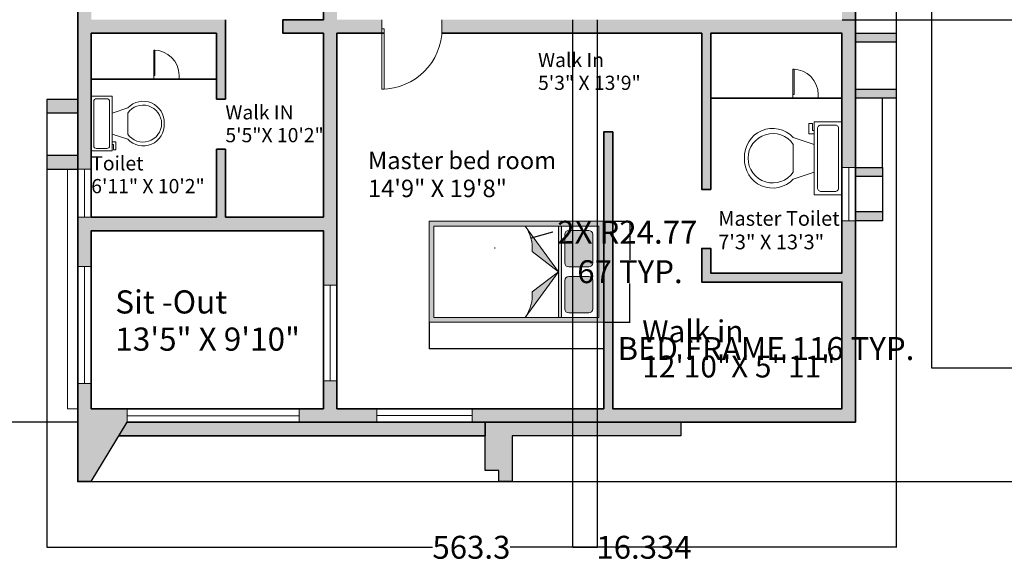
# Model space of a CAD drawing. Units: inches. Extents: x -828 to 1568, y -491 to 539.
# Tile 4 of 6: x 241 to 895, y -470 to -110. Entities that reach past the tile are written whole.
import ezdxf

# ---------------------------------------------------------------- set-up
doc = ezdxf.new("R2010")
doc.units = ezdxf.units.IN
doc.header["$MEASUREMENT"] = 0
doc.linetypes.add('ACAD_ISO02W100', pattern=[15, 12, -3])
for name, color, linetype, lineweight in [('A-ANNO-DIMS', 2, 'Continuous', 18), ('A-AREA-IDEN', 7, 'Continuous', 18), ('A-DOOR', 3, 'Continuous', 18), ('A-FLOR-EDGE', 7, 'Continuous', 25), ('A-FLOR-FIXT', 9, 'Continuous', 18), ('A-FLOR-OVHD', 116, 'ACAD_ISO02W100', 13), ('A-FLOR-SHFT', 7, 'Continuous', 25), ('A-FURN', 8, 'Continuous', 18), ('A-FURN-PATT', 253, 'Continuous', 13), ('A-GLAZ', 4, 'Continuous', 18), ('A-WALL', 7, 'Continuous', 35), ('A-WALL-PATT', 8, 'Continuous', 13)]:
    doc.layers.add(name, color=color, linetype=linetype, lineweight=lineweight)
doc.styles.get("Standard").update_dxf_attribs({"font": 'arial.ttf'})
doc.dimstyles.get("Standard").update_dxf_attribs({"dimtxt": 15.18, "dimasz": 0.18, "dimexe": 0.18, "dimexo": 0.0625, "dimgap": 0.09, "dimtad": 0, "dimtih": 1, "dimtoh": 1, "dimdec": 0, "dimzin": 0, "dimdsep": 46, "dimlunit": 3, "dimtxsty": 'Standard', "dimcen": 0.09, "dimadec": 0, "dimazin": 0, "dimtfac": 1, "dimtdec": 0, "dimtofl": 0, "dimtmove": 0, "dimatfit": 3, "dimfxl": 1, "dimtolj": 1, "dimtzin": 0, "dimarcsym": 0})

# ---------------------------------------------------------------- blocks, each defined once
blk = doc.blocks.new('*U2')
for p, q in [((0, 0), (0, -6)), ((40, 0), (40, -6))]:
    blk.add_line(p, q)
blk.add_lwpolyline([(0, 0), (0, 40), (1.75, 40), (1.75, 0)], close=True)
blk.add_arc((0, 0), 40, 0, 90)
blk = doc.blocks.new('*U6')
for p, q in [((9.5, -6), (9.5, -2)), ((-8, -8.5), (-8, -8)), ((-7, -8), (-7, -9.5)), ((-4, -8), (-6, -14)), ((4, -8), (6, -14)), ((-10, -8.5), (-8, -8.5)), ((-10, -9.5), (-10, -8.5)), ((-7, -9.5), (-10, -9.5)), ((4, -14), (-4, -14))]:
    blk.add_line(p, q)
blk.add_lwpolyline([(10.5, -8), (10.5, 0), (-10.5, 0), (-10.5, -8)], close=True)
for points in [[(-9.5, -2), (-9.5, -6)], [(8.5, -1), (-8.5, -1)], [(-8.5, -7), (8.5, -7)]]:
    blk.add_lwpolyline(points)
for centre, radius, start, end in [((-8.625, -1.875), 0.8839, 81.8699, 188.1301), ((8.625, -1.875), 0.8839, 351.8699, 98.1301), ((-8.625, -6.125), 0.8839, 171.869898, 278.1301), ((8.625, -6.125), 0.8839, 261.8699, 8.1301), ((-0.4772, -19.9188), 8.0953, 133.01722, 273.38), ((0.0374, -19.8731), 7.127, 124.50543, 269.7), ((-0.0373, -19.8731), 7.127, 270.3, 55.4946), ((0.4773, -19.9188), 8.0953, 266.62, 46.9828)]:
    blk.add_arc(centre, radius, start, end)
blk = doc.blocks.new('SERVICE-SHAFT-43')
blk.add_line((26.86, 37.12), (26.86, 6))
for points in [[(0, 43.12), (26.86, 43.12), (26.86, 37.12), (0, 37.12)], [(0, 6), (26.86, 6), (26.86, 0), (0, 0)]]:
    blk.add_lwpolyline(points, close=True)
blk = doc.blocks.new('BED-FRAME-TURNBACK')
h = blk.add_hatch(color=256)
h.dxf.hatch_style = 1
h.paths.add_polyline_path([(0, 0), (115.93, 0), (115.93, 67.12), (0, 67.12)])
h.paths.add_polyline_path([(3.27, 63.85), (112.66, 63.85), (112.66, 3.27), (3.27, 3.27)], flags=16)
h = blk.add_hatch(color=256)
h.dxf.hatch_style = 1
h.paths.add_polyline_path([(63.77, 63.85, -0.182673), (68.41, 46.96), (85.81, 33.56)])
h.paths.add_polyline_path([(85.81, 33.56), (68.41, 20.16, -0.182673), (63.77, 3.27)])
h = blk.add_hatch(color=256)
h.dxf.hatch_style = 1
h.paths.add_polyline_path([(87.78, 33.56), (85.81, 33.56), (85.81, 3.27), (87.78, 3.27)])
h.paths.add_polyline_path([(87.78, 63.85), (85.81, 63.85), (85.81, 33.56), (87.78, 33.56)])
for p, q in [((85.81, 33.56), (63.77, 63.85)), ((85.81, 3.27), (85.81, 63.85)), ((87.78, 3.27), (87.78, 63.85)), ((85.81, 33.56), (68.41, 46.96))]:
    blk.add_line(p, q)
for points in [[(115.93, 0), (0, 0), (0, 67.12), (115.93, 67.12)], [(112.66, 3.27), (3.27, 3.27), (3.27, 63.85), (112.66, 63.85)]]:
    blk.add_lwpolyline(points, close=True)
blk.add_lwpolyline([(63.77, 3.27, 0.182673), (68.41, 20.16), (85.81, 33.56)], format="xyb", close=True)
blk.add_arc((43.75, 49.27), 24.77, 354.63295, 36.04187)
blk = doc.blocks.new('*D29')
at = {"layer": 'A-ANNO-DIMS', "color": 0, "lineweight": -2, "transparency": 16777216}
for p, q in [((512.99, -311.15), (512.99, -328.66)), ((628.92, -311.15), (628.92, -328.66)), ((513.17, -328.48), (628.74, -328.48)), ((628.92, -328.48), (629.1, -328.48))]:
    blk.add_line(p, q, dxfattribs=at)
at = {"layer": 'A-ANNO-DIMS', "color": 0, "lineweight": 20, "transparency": 16777216}
for points in [[(513.17, -328.45), (513.17, -328.51), (512.99, -328.48)], [(628.74, -328.45), (628.74, -328.51), (628.92, -328.48)]]:
    blk.add_solid(points, dxfattribs=at)
at = {"layer": 'DEFPOINTS', "color": 0, "lineweight": 20, "transparency": 16777216}
for p in [(512.99, -311.09), (628.92, -311.09), (628.92, -328.48)]:
    blk.add_point(p, dxfattribs=at)
at = {"layer": 'A-ANNO-DIMS', "color": 0, "transparency": 16777216, "insert": (736.5, -328.48), "char_height": 15.18, "attachment_point": 5}
blk.add_mtext('\\A1;BED FRAME 116 TYP.', dxfattribs=at)
blk = doc.blocks.new('*D30')
at = {"layer": 'A-ANNO-DIMS', "color": 0, "lineweight": -2, "transparency": 16777216}
for p, q in [((628.99, -243.97), (646.49, -243.97)), ((646.31, -244.15), (646.31, -269.69)), ((646.31, -310.91), (646.31, -285.37)), ((628.99, -311.09), (646.49, -311.09))]:
    blk.add_line(p, q, dxfattribs=at)
at = {"layer": 'A-ANNO-DIMS', "color": 0, "lineweight": 20, "transparency": 16777216}
for points in [[(646.28, -244.15), (646.34, -244.15), (646.31, -243.97)], [(646.28, -310.91), (646.34, -310.91), (646.31, -311.09)]]:
    blk.add_solid(points, dxfattribs=at)
at = {"layer": 'DEFPOINTS', "color": 0, "lineweight": 20, "transparency": 16777216}
for p in [(628.92, -243.97), (646.31, -243.97), (628.92, -311.09)]:
    blk.add_point(p, dxfattribs=at)
at = {"layer": 'A-ANNO-DIMS', "color": 0, "transparency": 16777216, "insert": (646.31, -277.53), "char_height": 15.18, "attachment_point": 5}
blk.add_mtext('\\A1;67 TYP.', dxfattribs=at)
blk = doc.blocks.new('*D39')
at = {"layer": 'A-ANNO-DIMS', "color": 0, "lineweight": -2, "transparency": 16777216}
for p, q in [((822.78, -162.6), (822.78, -460.48)), ((259.43, -209.63), (259.43, -460.48)), ((259.61, -460.3), (515.4, -460.3)), ((822.6, -460.3), (566.81, -460.3))]:
    blk.add_line(p, q, dxfattribs=at)
at = {"layer": 'A-ANNO-DIMS', "color": 0, "lineweight": 20, "transparency": 16777216}
for points in [[(259.61, -460.27), (259.61, -460.33), (259.43, -460.3)], [(822.6, -460.27), (822.6, -460.33), (822.78, -460.3)]]:
    blk.add_solid(points, dxfattribs=at)
at = {"layer": 'DEFPOINTS', "color": 0, "lineweight": 20, "transparency": 16777216}
for p in [(822.78, -162.54), (259.43, -209.56), (822.78, -460.3)]:
    blk.add_point(p, dxfattribs=at)
at = {"layer": 'A-ANNO-DIMS', "color": 0, "transparency": 16777216, "insert": (541.11, -460.3), "char_height": 15.18, "attachment_point": 5}
blk.add_mtext('\\A1;563.3', dxfattribs=at)
blk = doc.blocks.new('*D40')
at = {"layer": 'A-ANNO-DIMS', "color": 0, "lineweight": -2, "transparency": 16777216}
for p, q in [((795.99, 360.63), (969.15, 360.63)), ((968.97, 360.45), (968.97, -20.38)), ((968.97, -416.57), (968.97, -35.74)), ((568.26, -416.75), (969.15, -416.75))]:
    blk.add_line(p, q, dxfattribs=at)
at = {"layer": 'A-ANNO-DIMS', "color": 0, "lineweight": 20, "transparency": 16777216}
for points in [[(968.94, 360.45), (969, 360.45), (968.97, 360.63)], [(968.94, -416.57), (969, -416.57), (968.97, -416.75)]]:
    blk.add_solid(points, dxfattribs=at)
at = {"layer": 'DEFPOINTS', "color": 0, "lineweight": 20, "transparency": 16777216}
for p in [(795.92, 360.63), (968.97, 360.63), (568.2, -416.75)]:
    blk.add_point(p, dxfattribs=at)
at = {"layer": 'A-ANNO-DIMS', "color": 0, "transparency": 16777216, "insert": (968.97, -28.06), "char_height": 15.18, "attachment_point": 5}
blk.add_mtext('\\A1;777.4', dxfattribs=at)
blk = doc.blocks.new('*D42')
at = {"layer": 'A-ANNO-DIMS', "color": 0, "lineweight": -2, "transparency": 16777216}
for p, q in [((347.86, 209.58), (141.48, 209.58)), ((141.66, 209.4), (141.66, -76.07)), ((141.66, -377.24), (141.66, -91.76)), ((279.86, -377.42), (141.48, -377.42))]:
    blk.add_line(p, q, dxfattribs=at)
at = {"layer": 'A-ANNO-DIMS', "color": 0, "lineweight": 20, "transparency": 16777216}
for points in [[(141.63, 209.4), (141.69, 209.4), (141.66, 209.58)], [(141.63, -377.24), (141.69, -377.24), (141.66, -377.42)]]:
    blk.add_solid(points, dxfattribs=at)
at = {"layer": 'DEFPOINTS', "color": 0, "lineweight": 20, "transparency": 16777216}
for p in [(141.66, 209.58), (347.92, 209.58), (279.92, -377.42)]:
    blk.add_point(p, dxfattribs=at)
at = {"layer": 'A-ANNO-DIMS', "color": 0, "transparency": 16777216, "insert": (141.66, -83.92), "char_height": 15.18, "attachment_point": 5}
blk.add_mtext('\\A1;587', dxfattribs=at)
blk = doc.blocks.new('*D47')
at = {"layer": 'A-ANNO-DIMS', "color": 0, "lineweight": -2, "transparency": 16777216}
for p, q in [((786.99, -22.42), (969.15, -22.42)), ((968.97, -22.6), (968.97, -58.57)), ((968.97, -110.24), (968.97, -74.26)), ((786.99, -110.42), (969.15, -110.42))]:
    blk.add_line(p, q, dxfattribs=at)
at = {"layer": 'A-ANNO-DIMS', "color": 0, "lineweight": 20, "transparency": 16777216}
for points in [[(968.94, -22.6), (969, -22.6), (968.97, -22.42)], [(968.94, -110.24), (969, -110.24), (968.97, -110.42)]]:
    blk.add_solid(points, dxfattribs=at)
at = {"layer": 'DEFPOINTS', "color": 0, "lineweight": 20, "transparency": 16777216}
for p in [(786.92, -22.42), (968.97, -22.42), (786.92, -110.42)]:
    blk.add_point(p, dxfattribs=at)
at = {"layer": 'A-ANNO-DIMS', "color": 0, "transparency": 16777216, "insert": (968.97, -66.42), "char_height": 15.18, "attachment_point": 5}
blk.add_mtext('\\A1;88', dxfattribs=at)
blk = doc.blocks.new('*D48')
at = {"layer": 'A-ANNO-DIMS', "color": 0, "lineweight": -2, "transparency": 16777216}
for p, q in [((608.26, -110.48), (608.26, -460.48)), ((624.59, -110.48), (624.59, -460.48)), ((608.44, -460.3), (624.41, -460.3)), ((624.59, -460.3), (624.77, -460.3))]:
    blk.add_line(p, q, dxfattribs=at)
at = {"layer": 'A-ANNO-DIMS', "color": 0, "lineweight": 20, "transparency": 16777216}
for points in [[(608.44, -460.27), (608.44, -460.33), (608.26, -460.3)], [(624.41, -460.27), (624.41, -460.33), (624.59, -460.3)]]:
    blk.add_solid(points, dxfattribs=at)
at = {"layer": 'DEFPOINTS', "color": 0, "lineweight": 20, "transparency": 16777216}
for p in [(608.26, -110.42), (624.59, -110.42), (624.59, -460.3)]:
    blk.add_point(p, dxfattribs=at)
at = {"layer": 'A-ANNO-DIMS', "color": 0, "transparency": 16777216, "insert": (655.62, -460.3), "char_height": 15.18, "attachment_point": 5}
blk.add_mtext('\\A1;16.334', dxfattribs=at)
blk = doc.blocks.new('*D54')
at = {"layer": 'A-ANNO-DIMS', "color": 0, "lineweight": -2, "transparency": 16777216}
for p, q in [((1093.6, 227.56), (846.26, 227.56)), ((846.44, 227.38), (846.44, -49.1)), ((846.44, -341.26), (846.44, -64.78)), ((1093.6, -341.44), (846.26, -341.44))]:
    blk.add_line(p, q, dxfattribs=at)
at = {"layer": 'A-ANNO-DIMS', "color": 0, "lineweight": 20, "transparency": 16777216}
for points in [[(846.41, 227.38), (846.47, 227.38), (846.44, 227.56)], [(846.41, -341.26), (846.47, -341.26), (846.44, -341.44)]]:
    blk.add_solid(points, dxfattribs=at)
at = {"layer": 'DEFPOINTS', "color": 0, "lineweight": 20, "transparency": 16777216}
for p in [(846.44, 227.56), (1093.66, 227.56), (1093.66, -341.44)]:
    blk.add_point(p, dxfattribs=at)
at = {"layer": 'A-ANNO-DIMS', "color": 0, "transparency": 16777216, "insert": (846.44, -56.94), "char_height": 15.18, "attachment_point": 5}
blk.add_mtext('\\A1;569', dxfattribs=at)
blk = doc.blocks.new('*D56')
at = {"layer": 'A-ANNO-DIMS', "color": 0, "lineweight": -2, "transparency": 16777216}
for p, q in [((594.95, -251.33), (580.8, -255.22)), ((595.13, -251.33), (594.95, -251.33)), ((556.64, -261.82), (556.82, -261.82)), ((556.73, -261.91), (556.73, -261.73))]:
    blk.add_line(p, q, dxfattribs=at)
at = {"layer": 'A-ANNO-DIMS', "color": 0, "lineweight": 20, "transparency": 16777216}
blk.add_solid([(580.79, -255.19), (580.8, -255.25), (580.62, -255.27)], dxfattribs=at)
at = {"layer": 'DEFPOINTS', "color": 0, "lineweight": 20, "transparency": 16777216}
for p in [(580.62, -255.27), (556.73, -261.82)]:
    blk.add_point(p, dxfattribs=at)
at = {"layer": 'A-ANNO-DIMS', "color": 0, "transparency": 16777216, "insert": (644.54, -251.33), "char_height": 15.18, "attachment_point": 5}
blk.add_mtext('\\A1;2X R24.77', dxfattribs=at)

msp = doc.modelspace()

# ---------------------------------------------------------------- hatches: boundary and pattern name
at = {"layer": 'A-FURN-PATT'}
h = msp.add_hatch(color=256, dxfattribs=at)
h.dxf.hatch_style = 1
h.paths.add_polyline_path([(621.5603, -252.8382, 0.41421356), (618.9442, -250.2221), (605.6981, -250.2221, 0.41421356), (603.0819, -252.8382), (603.0819, -271.7144, 0.41421356), (605.6981, -274.3306), (618.9442, -274.3306, 0.41421356), (621.5603, -271.7144)])
h = msp.add_hatch(color=256, dxfattribs=at)
h.dxf.hatch_style = 1
h.paths.add_polyline_path([(603.0819, -302.2257, 0.41421356), (605.6981, -304.8418), (618.9442, -304.8418, 0.41421356), (621.5603, -302.2257), (621.5603, -283.3495, 0.41421356), (618.9442, -280.7333), (605.6981, -280.7333, 0.41421356), (603.0819, -283.3495)])
at = {"layer": 'A-WALL-PATT'}
h = msp.add_hatch(color=256, dxfattribs=at)
h.dxf.hatch_style = 1
h.paths.add_polyline_path([(795.9226, -243.7164), (786.9226, -243.7164), (786.9226, -278.4155), (699.9226, -278.4155), (699.9226, -262.0576), (693.9226, -262.0576), (693.9226, -284.4155), (786.9226, -284.4155), (786.9226, -368.4155), (634.9226, -368.4155), (634.9226, -184.8338), (628.9226, -184.8338), (628.9226, -368.4155), (541.609, -368.4155), (541.609, -377.4155), (795.9226, -377.4155)])
h.paths.add_polyline_path([(795.9226, -80.4153), (786.9226, -80.4153), (786.9226, -110.4155), (521.5942, -110.4155), (521.5942, -116.4155, -0.01876983), (521.4815, -119.4155), (693.9226, -119.4155), (693.9226, -222.9922), (699.9226, -222.9922), (699.9226, -119.4155), (786.9226, -119.4155), (786.9226, -208.3743), (795.9226, -208.3743)])
h.paths.add_polyline_path([(822.7802, -119.4155), (795.9226, -119.4155), (795.9226, -125.4155), (822.7802, -125.4155)])
h.paths.add_polyline_path([(822.7802, -80.4153), (795.9226, -80.4153), (795.9226, -86.4153), (822.7802, -86.4153)])
h.paths.add_polyline_path([(822.7802, -156.5366), (795.9226, -156.5366), (795.9226, -162.5366), (822.7802, -162.5366)])
h.paths.add_polyline_path([(813.7802, -208.3743), (795.9226, -208.3743), (795.9226, -214.3743), (813.7802, -214.3743)])
h.paths.add_polyline_path([(813.7802, -237.7164), (795.9226, -237.7164), (795.9226, -243.7164), (813.7802, -243.7164)])
h.paths.add_polyline_path([(568.196, -386.4155), (680.1012, -386.4155), (680.1012, -377.4155), (550.196, -377.4155), (550.196, -409.2892), (559.196, -409.2892), (559.196, -416.7473), (568.196, -416.7473)])
h.paths.add_polyline_path([(478.3036, -368.4155), (451.9226, -368.4155), (451.9226, -349.8576), (442.9226, -349.8576), (442.9226, -368.4155), (426.7914, -368.4155), (426.7914, -377.4155), (478.3036, -377.4155)])
h.paths.add_polyline_path([(550.196, -377.4155), (541.609, -377.4155), (426.7914, -377.4155), (426.7914, -377.6482), (312.8078, -377.4155), (307.3423, -386.4155), (550.196, -386.4155)])
h.paths.add_polyline_path([(312.8078, -377.4155), (312.8078, -368.4155), (288.9226, -368.4155), (288.9226, -351.7781), (279.9226, -351.7781), (279.9226, -377.4155), (279.9226, -416.7473), (288.9226, -416.7473)])
h.paths.add_polyline_path([(451.9226, -119.4155), (481.5942, -119.4155), (481.5942, -116.4155), (481.5942, -110.4155), (451.9226, -110.4155), (451.9226, -5.2313), (445.9226, -5.2313, -0.01876983), (442.9226, -5.1187), (442.9226, -110.4155), (416.0227, -110.4155), (416.0227, -119.4155), (442.9226, -119.4155), (442.9226, -241.4155), (377.9226, -241.4155), (377.9226, -196.3369), (371.9226, -196.3369), (371.9226, -241.4155), (288.9226, -241.4155), (279.9226, -241.4155), (279.9226, -273.9916), (288.9226, -273.9916), (288.9226, -250.4155), (442.9226, -250.4155), (442.9226, -286.5741), (451.9226, -286.5741)])
h.paths.add_polyline_path([(377.9226, -110.4155), (288.9226, -110.4155), (288.9226, -23.5133), (279.9226, -23.5133), (279.9226, -209.5643), (288.9226, -209.5643), (288.9226, -119.4155), (371.9226, -119.4155), (371.9226, -163.1368), (377.9226, -163.1368)], flags=17)
h.paths.add_polyline_path([(279.9226, -200.5643), (259.4345, -200.5643), (259.4345, -209.5643), (279.9226, -209.5643)])
h.paths.add_polyline_path([(279.9226, -163.4155), (259.4345, -163.4155), (259.4345, -172.4155), (279.9226, -172.4155)])
h.paths.add_polyline_path([(680.9226, 59.5845), (569.9226, 59.5845), (569.9226, 238.5845), (603.4634, 238.5845), (603.4634, 244.5845), (569.9226, 244.5845), (569.9226, 333.5845), (663.9226, 333.5845), (663.9226, 280.6911), (667.9428, 280.6911, -0.00914136), (668.9226, 280.6732), (668.9226, 333.5845), (696.1553, 333.5845), (696.1553, 342.5845), (560.9226, 342.5845), (560.9226, 333.5845), (560.9226, 229.5845), (560.9226, 212.3675), (560.9226, 207.5845), (560.9226, 59.5845), (347.9226, 59.5845), (347.9226, 75.0877), (338.9226, 75.0877), (338.9226, 59.5845), (279.9226, 59.5845), (279.9226, 50.5845), (288.9226, 50.5845), (442.9226, 50.5845), (442.9226, 34.7687), (445.9226, 34.7687), (451.9226, 34.7687), (451.9226, 50.5845), (591.9226, 50.5845), (591.9226, 37.5639), (600.9226, 37.5639), (600.9226, 50.5845), (671.9226, 50.5845), (671.9226, -13.4155), (600.9226, -13.4155), (600.9226, -1.0868), (591.9226, -1.0868), (591.9226, -22.4155), (680.9226, -22.4155), (786.9226, -22.4155), (786.9226, -13.4155), (680.9226, -13.4155)])
h.paths.add_polyline_path([(813.7802, -22.4155), (795.9226, -22.4155), (795.9226, -28.4155), (813.7802, -28.4155)])
h.paths.add_polyline_path([(795.9226, 59.5845), (786.9226, 59.5845), (786.9226, -13.4155), (786.9226, -22.4155), (786.9226, -28.4155), (795.9226, -28.4155), (795.9226, -22.4155)])
h.paths.add_polyline_path([(813.7802, 16.5847), (795.9226, 16.5847), (795.9226, 10.5847), (813.7802, 10.5847)])
h.paths.add_polyline_path([(795.9226, 342.5845), (791.2302, 342.5845), (738.4317, 342.5845), (738.4317, 333.5845), (786.9226, 333.5845), (786.9226, 244.5845), (668.9226, 244.5845), (668.9226, 253.8895), (667.9428, 253.8895), (663.9226, 253.8895), (663.9226, 244.5845), (645.6004, 244.5845), (645.6004, 238.5845), (786.9226, 238.5845), (786.9226, 144.7189), (795.9226, 144.7189)])
h.paths.add_polyline_path([(822.7802, 207.4634), (795.9226, 207.4634), (795.9226, 201.4634), (822.7802, 201.4634)])
h.paths.add_polyline_path([(822.7802, 244.5845), (795.9226, 244.5845), (795.9226, 238.5845), (822.7802, 238.5845)])
h.paths.add_polyline_path([(347.9226, 207.5845), (386.8215, 207.5845), (485.9226, 207.5845), (485.9226, 229.5845), (489.9226, 229.5845), (489.9226, 244.2539), (489.9226, 333.5845), (521.5185, 333.5845), (521.5185, 342.5845), (279.9226, 342.5845), (279.9226, 333.5845), (338.9226, 333.5845), (347.9226, 333.5845), (483.9226, 333.5845), (483.9226, 209.5845), (386.8215, 209.5845), (338.9226, 209.5845), (279.9226, 209.5845), (279.9226, 200.5845), (288.9226, 200.5845), (338.9226, 200.5845), (338.9226, 180.8391), (347.9226, 180.8391)])
h.paths.add_polyline_path([(795.9226, 360.6319), (791.2302, 360.6319), (791.2302, 342.5845), (795.9226, 342.5845)])
h.paths.add_polyline_path([(755.2954, 360.6319), (750.6031, 360.6319), (750.6031, 342.5845), (755.2954, 342.5845)])
h.paths.add_polyline_path([(738.4317, 352.9518), (732.1778, 352.9518), (732.1778, 342.5845), (738.4317, 342.5845)])
h.paths.add_polyline_path([(702.4092, 352.9518), (696.1553, 352.9518), (696.1553, 342.5845), (702.4092, 342.5845)])
h.paths.add_polyline_path([(475.4018, 360.6319), (470.7095, 360.6319), (470.7095, 342.5845), (475.4018, 342.5845)])
h.paths.add_polyline_path([(448.7297, 360.6319), (444.0374, 360.6319), (444.0374, 342.5845), (448.7297, 342.5845)])
h.paths.add_polyline_path([(489.9226, 229.5845), (485.9226, 229.5845), (485.9226, 207.5845), (489.9226, 207.5845), (489.9226, 212.3675)], flags=17)
h.paths.add_polyline_path([(708.7018, -15.9815), (795.2211, -15.9815), (795.2211, -1.5493), (708.7018, -1.5493)], flags=9)
h.paths.add_polyline_path([(598.5172, 15.6725), (685.0365, 15.6725), (685.0365, 30.1047), (598.5172, 30.1047)], flags=25)
h.paths.add_polyline_path([(598.5188, 30.8165), (677.2194, 30.8165), (677.2194, 45.2391), (598.5188, 45.2391)], flags=25)

# ---------------------------------------------------------------- linework, layer by layer
at = {"layer": 'A-FLOR-EDGE'}
for p, q in [((288.9226, -416.7473), (312.8078, -377.4155)), ((550.196, -409.2892), (550.196, -377.4155)), ((559.196, -409.2892), (550.196, -409.2892)), ((559.196, -416.7473), (559.196, -409.2892)), ((288.9226, -416.7473), (568.196, -416.7473)), ((568.196, -416.7473), (559.196, -416.7473))]:
    msp.add_line(p, q, dxfattribs=at)
for points in [[(550.196, -377.4155), (550.196, -386.4155)], [(307.3423, -386.4155), (550.196, -386.4155)]]:
    msp.add_lwpolyline(points, close=True, dxfattribs=at)
msp.add_lwpolyline([(680.1012, -377.4155), (680.1012, -386.4155), (568.196, -386.4155), (568.196, -416.7473)], dxfattribs=at)
at = {"layer": 'A-FLOR-OVHD'}
msp.add_lwpolyline([(273.1806, -368.4155), (273.1806, -209.5643), (273.1806, -368.4155), (279.9226, -368.4155)], dxfattribs=at)
at = {"layer": 'A-FLOR-SHFT'}
for p, q in [((822.7802, -86.4153), (822.7802, -119.4155)), ((813.7802, -208.3743), (813.7802, -162.5366)), ((279.9226, -200.5643), (259.4345, -200.5643)), ((813.7802, -214.3743), (813.7802, -237.7164))]:
    msp.add_line(p, q, dxfattribs=at)
for points in [[(279.9226, -163.4155), (259.4345, -163.4155), (259.4345, -172.4155)], [(279.9226, -172.4155), (259.4345, -172.4155), (259.4345, -200.5643), (259.4345, -209.5643), (279.9226, -209.5643)], [(786.9226, -214.3743), (786.9226, -208.3743)], [(795.9226, -208.3743), (813.7802, -208.3743), (813.7802, -214.3743), (795.9226, -214.3743)], [(786.9226, -243.7164), (786.9226, -237.7164)], [(795.9226, -237.7164), (813.7802, -237.7164), (813.7802, -243.7164), (795.9226, -243.7164)]]:
    msp.add_lwpolyline(points, dxfattribs=at)
at = {"layer": 'A-FURN'}
for points in [[(618.9442, -274.3306), (605.6981, -274.3306, -0.41421356), (603.0819, -271.7144), (603.0819, -252.8382, -0.41421356), (605.6981, -250.2221), (618.9442, -250.2221, -0.41421356), (621.5603, -252.8382), (621.5603, -271.7144, -0.41421356)], [(618.9442, -280.7333), (605.6981, -280.7333, 0.41421356), (603.0819, -283.3495), (603.0819, -302.2257, 0.41421356), (605.6981, -304.8418), (618.9442, -304.8418, 0.41421356), (621.5603, -302.2257), (621.5603, -283.3495, 0.41421356)]]:
    msp.add_lwpolyline(points, format="xyb", close=True, dxfattribs=at)
at = {"layer": 'A-GLAZ'}
for p, q in [((791.4226, -243.7164), (791.4226, -208.3743)), ((284.4226, -241.4155), (284.4226, -209.5643)), ((284.4226, -351.7781), (284.4226, -273.9916)), ((447.4226, -349.8576), (447.4226, -286.5741)), ((426.7914, -373.1482), (312.8078, -373.1482)), ((541.609, -372.9155), (478.3036, -372.9155))]:
    msp.add_line(p, q, dxfattribs=at)
for points in [[(795.9226, -243.7164), (786.9226, -243.7164), (786.9226, -208.3743), (795.9226, -208.3743)], [(288.9226, -241.4155), (279.9226, -241.4155), (279.9226, -209.5643), (288.9226, -209.5643)], [(288.9226, -351.7781), (279.9226, -351.7781), (279.9226, -273.9916), (288.9226, -273.9916)], [(451.9226, -349.8576), (442.9226, -349.8576), (442.9226, -286.5741), (451.9226, -286.5741)], [(312.8078, -377.4155), (426.7914, -377.6482), (426.7914, -368.6482), (312.8078, -368.4155)], [(478.3036, -368.4155), (541.609, -368.4155), (541.609, -377.4155), (478.3036, -377.4155)]]:
    msp.add_lwpolyline(points, close=True, dxfattribs=at)
at = {"layer": 'A-WALL'}
for p, q in [((795.9226, 342.5845), (795.9226, -377.4155)), ((377.9226, -163.1368), (377.9226, -110.4155)), ((288.9226, -119.4155), (371.9226, -119.4155)), ((288.9226, -119.4155), (288.9226, -241.4155)), ((288.9226, -241.4155), (288.9226, -119.4155)), ((371.9226, -163.1368), (371.9226, -119.4155)), ((442.9226, -119.4155), (442.9226, -241.4155)), ((288.9226, -149.8674), (371.9226, -149.8674)), ((699.9226, -162.5366), (786.9226, -162.5366)), ((371.9226, -241.4155), (371.9226, -196.3369)), ((377.9226, -241.4155), (377.9226, -196.3369)), ((288.9226, -241.4155), (371.9226, -241.4155)), ((377.9226, -241.4155), (442.9226, -241.4155)), ((312.8078, -377.4155), (795.9226, -377.4155))]:
    msp.add_line(p, q, dxfattribs=at)
for points in [[(279.9226, 333.5845), (279.9226, 342.5845), (279.9226, 50.5845), (279.9226, -377.4155), (279.9226, -416.7473), (288.9226, -416.7473)], [(442.9226, -241.4155), (442.9226, -119.4155), (416.0227, -119.4155), (416.0227, -110.4155), (442.9226, -110.4155), (442.9226, -5.1187)], [(786.9226, -119.4155), (699.9226, -119.4155), (786.9226, -119.4155), (786.9226, -278.4155), (699.9226, -278.4155), (699.9226, -262.0576), (693.9226, -262.0576), (693.9226, -284.4155), (786.9226, -284.4155), (786.9226, -368.4155), (634.9226, -368.4155), (634.9226, -184.8338), (628.9226, -184.8338), (628.9226, -368.4155), (451.9226, -368.4155), (451.9226, -119.4155), (483.3442, -119.4155)], [(521.4815, -119.4155), (693.9226, -119.4155), (693.9226, -222.9922), (699.9226, -222.9922), (699.9226, -119.4155)], [(371.9226, -163.1368), (377.9226, -163.1368)], [(377.9226, -196.3369), (371.9226, -196.3369)]]:
    msp.add_lwpolyline(points, dxfattribs=at)
msp.add_lwpolyline([(288.9226, -368.4155), (442.9226, -368.4155), (442.9226, -250.4155), (288.9226, -250.4155)], close=True, dxfattribs=at)

# ---------------------------------------------------------------- block references
at = {"layer": 'A-DOOR', "xscale": -1, "rotation": 180}
msp.add_blockref('*U2', (481.5942, -116.4155), dxfattribs=at)
at = {"layer": 'A-DOOR', "xscale": 0.4187164315817437, "yscale": 0.4187164315817437, "zscale": 0.4187164315817437}
for p in [(330.4226, -147.3551), (754.4226, -160.0243)]:
    msp.add_blockref('*U2', p, dxfattribs=at)
at = {"layer": 'A-FLOR-FIXT'}
for p, xscale, yscale, zscale, rotation in [((288.9226, -179.3229), 1.728531319999881, 1.728531319999881, 1.728531319999881, 90), ((786.9226, -202.3123), 2.308307865517238, 2.308307865517238, 2.308307865517238, 270)]:
    msp.add_blockref('*U6', p, dxfattribs=dict(at, xscale=xscale, yscale=yscale, zscale=zscale, rotation=rotation))
at = {"layer": 'A-FLOR-SHFT'}
msp.add_blockref('SERVICE-SHAFT-43', (795.923, -162.537), dxfattribs=at)
at = {"layer": 'A-FURN'}
msp.add_blockref('BED-FRAME-TURNBACK', (512.989, -311.0915), dxfattribs=at)

# ---------------------------------------------------------------- texts
at = {"layer": 'A-AREA-IDEN'}
for s, height, p in [('Walk In', 9.42222, (585.3115, -141.8405)), ('5\'3" X 13\'9"', 9.422225, (585.3115, -156.9765)), ('Walk IN', 9.42222, (377.9226, -176.5448)), ('5\'5"X 10\'2"', 9.422225, (377.9226, -191.6808)), ('Toilet ', 9.42222, (288.9226, -210.3539)), ('Master bed room', 11.542757, (472.4915, -209.5342)), ('6\'11" X 10\'2"', 9.422225, (288.9226, -225.4899)), ('14\'9" X 19\'8"', 11.542757, (472.4915, -228.0766)), ('Master Toilet', 9.717003, (704.8376, -247.0736)), ('7\'3" X 13\'3"', 9.717003, (704.8376, -262.6831)), ('Sit -Out', 15.34207, (304.876, -305.2596)), ('Walk in', 14.539, (654.4439, -324.3313)), ('13\'5" X 9\'10"', 15.34207, (304.876, -329.9053)), ('12\'10"X 5\'\'11"', 14.538996, (654.4439, -347.687))]:
    msp.add_text(s, height=height, dxfattribs=at).set_placement(p)

# ---------------------------------------------------------------- dimensions: what is measured, and where the dimension line sits
at = {"layer": 'A-ANNO-DIMS'}
for base, p1, p2, override, picture, middle in [((968.971, 360.6319), (568.196, -416.7473), (795.9226, 360.6319), {"dimdec": 1, "dimlfac": 1, "dimrnd": 0, "dimzin": 0, "dimdsep": 46, "dimlunit": 2}, '*D40', (968.971, -28.0577)), ((846.4381, 227.5603), (1093.6584, -341.4397), (1093.6584, 227.5603), {"dimdec": 0, "dimlfac": 1, "dimrnd": 0, "dimzin": 0, "dimdsep": 46, "dimlunit": 2}, '*D54', (846.4381, -56.9397)), ((141.6607, 209.5845), (279.9226, -377.4155), (347.9226, 209.5845), {"dimdec": 0, "dimlfac": 1, "dimrnd": 0, "dimzin": 0, "dimdsep": 46, "dimlunit": 2}, '*D42', (141.6607, -83.9155)), ((968.971, -22.4155), (786.9226, -110.4155), (786.9226, -22.4155), {"dimdec": 0, "dimlfac": 1, "dimrnd": 0, "dimzin": 0, "dimdsep": 46, "dimlunit": 2}, '*D47', (968.971, -66.4155))]:
    dim = msp.add_linear_dim(base=base, p1=p1, p2=p2, angle=90, dimstyle='Standard', override=override, dxfattribs=at)
    dim.commit()
    dim.dimension.update_dxf_attribs({"geometry": picture, "text_midpoint": middle})
for base, p1, p2, override, picture, middle in [((624.589571, -460.297328), (608.256067, -110.415466), (624.589571, -110.415466), {"dimdec": 3, "dimlfac": 1, "dimrnd": 0, "dimzin": 0, "dimdsep": 46, "dimlunit": 2}, '*D48', (655.623405, -460.297328)), ((822.7802, -460.2973), (259.4345, -209.5643), (822.7802, -162.5366), {"dimdec": 1, "dimlfac": 1, "dimrnd": 0, "dimzin": 0, "dimdsep": 46, "dimlunit": 2}, '*D39', (541.1073, -460.2973))]:
    dim = msp.add_linear_dim(base=base, p1=p1, p2=p2, dimstyle='Standard', override=override, dxfattribs=at)
    dim.commit()
    dim.dimension.update_dxf_attribs({"geometry": picture, "text_midpoint": middle})
dim = msp.add_radius_dim(center=(556.7345, -261.8166), mpoint=(580.6216, -255.2651), text='2X <>', dimstyle='Standard', override={"dimdec": 2, "dimlfac": 1, "dimrnd": 0, "dimzin": 0, "dimdsep": 46, "dimlunit": 2}, dxfattribs=at)
dim.commit()
dim.dimension.update_dxf_attribs({"geometry": '*D56', "text_midpoint": (644.5382, -251.3342), "dimtype": 164})
dim = msp.add_linear_dim(base=(646.3125, -243.9728), p1=(628.9226, -311.0911), p2=(628.9226, -243.9728), angle=90, text='<> TYP.', dimstyle='Standard', override={"dimdec": 0, "dimlfac": 1, "dimrnd": 0, "dimzin": 0, "dimdsep": 46, "dimlunit": 2}, dxfattribs=at)
dim.commit()
dim.dimension.update_dxf_attribs({"geometry": '*D30', "text_midpoint": (646.3125, -277.532)})
dim = msp.add_linear_dim(base=(628.9226, -328.4811), p1=(512.9895, -311.0911), p2=(628.9226, -311.0911), text='BED FRAME <> TYP.', dimstyle='Standard', override={"dimdec": 0, "dimlfac": 1, "dimrnd": 0, "dimzin": 0, "dimdsep": 46, "dimlunit": 2}, dxfattribs=at)
dim.commit()
dim.dimension.update_dxf_attribs({"geometry": '*D29', "text_midpoint": (736.5036, -328.4811)})

doc.saveas('drawing.dxf')
